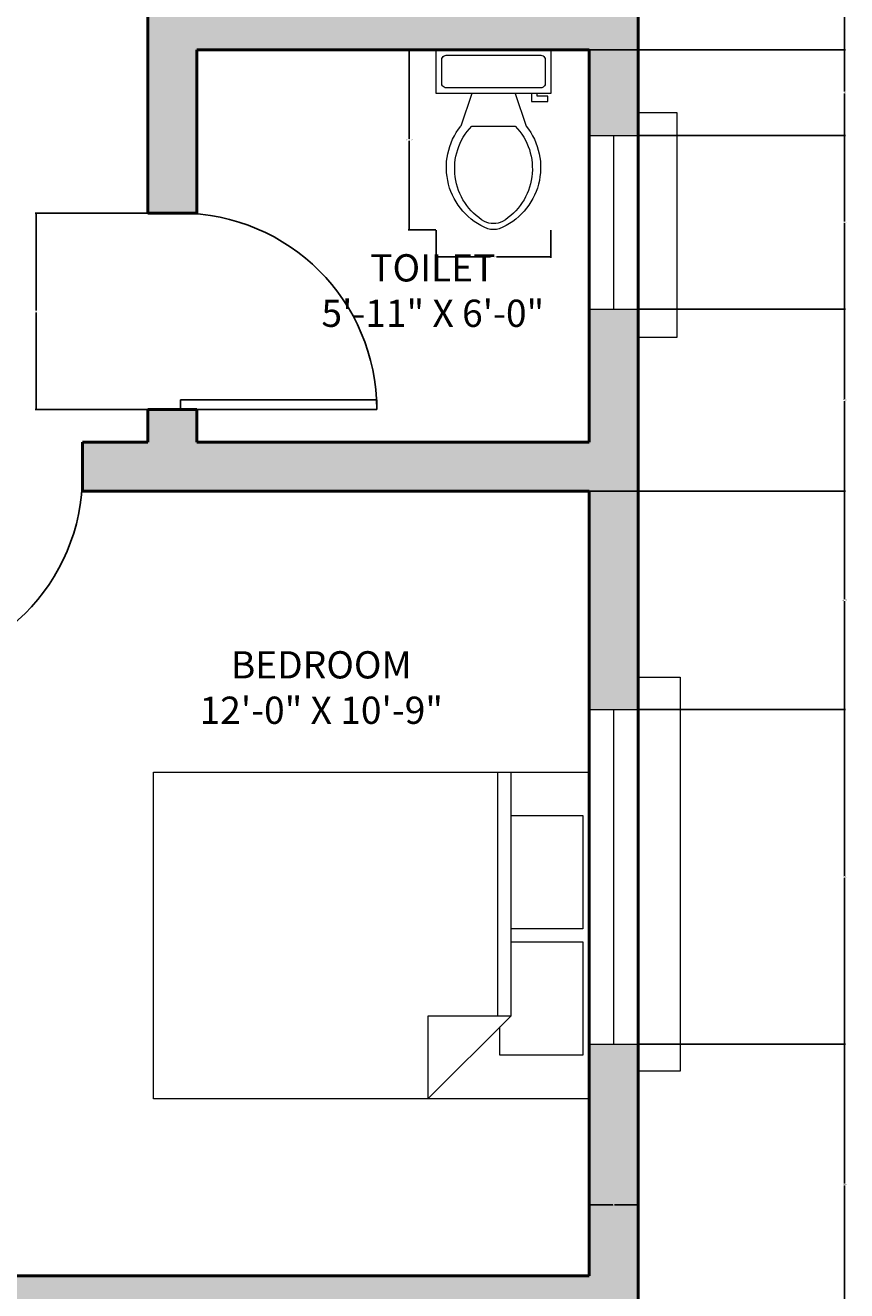
# Model space of a CAD drawing. Units: inches. Extents: x 2710 to 3197, y 524 to 1147.
# Tile 4 of 6: x 3046 to 3197, y 640 to 873. Entities that reach past the tile are written whole.
import ezdxf

# ---------------------------------------------------------------- set-up
doc = ezdxf.new("R2010")
doc.units = ezdxf.units.IN
for name, color, linetype, lineweight in [('A-ANNO-DIMS', 2, 'Continuous', 18), ('A-AREA-IDEN', 7, 'Continuous', 25), ('A-DOOR', 3, 'Continuous', 25), ('A-FLOR-FIXT', 9, 'Continuous', 20), ('A-FURN', 8, 'Continuous', 18), ('A-GLAZ', 4, 'Continuous', 18), ('A-WALL', 7, 'Continuous', 50), ('A-WALL-PATT', 74, 'Continuous', 13)]:
    doc.layers.add(name, color=color, linetype=linetype, lineweight=lineweight)
doc.styles.get("Standard").update_dxf_attribs({"font": 'arial.ttf'})
doc.dimstyles.get("Standard").update_dxf_attribs({"dimtxt": 0.18, "dimasz": 0.18, "dimexe": 0.18, "dimexo": 0.0625, "dimgap": 0.09, "dimtad": 0, "dimtih": 1, "dimtoh": 1, "dimdec": 4, "dimzin": 0, "dimdsep": 46, "dimtxsty": 'Standard', "dimcen": 0.09, "dimadec": 0, "dimazin": 0, "dimtfac": 1, "dimtdec": 4, "dimtofl": 0, "dimtmove": 0, "dimatfit": 3, "dimfxl": 1, "dimtolj": 1, "dimtzin": 0, "dimarcsym": 0})

# ---------------------------------------------------------------- blocks, each defined once
blk = doc.blocks.new('*U8')
for p, q in [((0, 0), (0, 6)), ((36, 0), (36, 6))]:
    blk.add_line(p, q)
blk.add_lwpolyline([(0, 0), (0, -36), (1.75, -36), (1.75, 0)], close=True)
blk.add_arc((0, 0), 36, 270, 0)
blk = doc.blocks.new('*U10')
for p, q in [((0, 0), (0, -6)), ((-36, 0), (-36, -6))]:
    blk.add_line(p, q)
blk.add_lwpolyline([(0, 0), (0, 36), (-1.75, 36), (-1.75, 0)], close=True)
blk.add_arc((0, 0), 36, 90, 180)
blk = doc.blocks.new('Bed - Queen')
for p, q in [((0, -80.00003), (0, 0)), ((0, 0), (59.99999, 0)), ((59.99999, 0), (59.99999, -80.00003)), ((7.99999, -1.2), (28.79998, -1.2)), ((7.99999, -14.4), (7.99999, -1.2)), ((28.79998, -1.2), (28.79998, -14.4)), ((31.19999, -1.2), (51.99999, -1.2)), ((31.19999, -14.4), (31.19999, -1.2)), ((51.99999, -1.2), (51.99999, -16.4)), ((0, -14.4), (44.8, -14.4)), ((59.99999, -29.6), (44.8, -14.4)), ((44.8, -14.4), (44.8, -29.6)), ((44.8, -16.8), (0, -16.8)), ((51.99999, -16.4), (46.79936, -16.4)), ((44.8, -29.6), (59.99999, -29.6)), ((59.99999, -80.00003), (0, -80.00003))]:
    blk.add_line(p, q)
blk = doc.blocks.new('Toilet - top')
for p, q in [((9.5, -6), (9.5, -2)), ((-10, -8.5), (-8, -8.5)), ((-10, -9.5), (-10, -8.5)), ((-8, -8.5), (-8, -8)), ((-7, -8), (-7, -9.5)), ((-4, -8), (-6, -14)), ((4, -8), (6, -14)), ((-7, -9.5), (-10, -9.5)), ((4, -14), (-4, -14))]:
    blk.add_line(p, q)
blk.add_lwpolyline([(10.5, -8), (10.5, 0), (-10.5, 0), (-10.5, -8)], close=True)
for points in [[(-9.5, -2), (-9.5, -6)], [(8.5, -1), (-8.5, -1)], [(-8.5, -7), (8.5, -7)]]:
    blk.add_lwpolyline(points)
for centre, radius, start, end in [((-8.62, -1.88), 0.884, 81.8699, 188.1301), ((8.62, -1.88), 0.884, 351.8699, 98.1301), ((-8.62, -6.12), 0.884, 171.8699, 278.1301), ((8.62, -6.12), 0.884, 261.8699, 8.1301), ((3.52, -21.58), 12.17, 141.4691, 247.9714), ((4.2, -21.82), 11.33, 136.3677, 238.9468), ((-3.52, -21.58), 12.17, 292.0284, 38.5307), ((-4.2, -21.82), 11.33, 301.053, 43.6321), ((0, -27.88), 4, 245.7318, 294.2682), ((0, -29), 4, 254.8605, 285.1395)]:
    blk.add_arc(centre, radius, start, end)
blk = doc.blocks.new('*D24')
at = {"layer": 'A-ANNO-DIMS', "color": 0, "lineweight": -2, "transparency": 16777216}
for p, q in [((3121.22, 868), (3116.14, 868)), ((3116.32, 867.82), (3116.32, 851.66)), ((3116.32, 835.14), (3116.32, 851.3)), ((3121.22, 834.96), (3116.14, 834.96))]:
    blk.add_line(p, q, dxfattribs=at)
at = {"layer": 'A-ANNO-DIMS', "color": 0, "transparency": 16777216}
for points in [[(3116.29, 867.82), (3116.35, 867.82), (3116.32, 868)], [(3116.29, 835.14), (3116.35, 835.14), (3116.32, 834.96)]]:
    blk.add_solid(points, dxfattribs=at)
at = {"layer": 'Defpoints', "color": 0, "transparency": 16777216}
for p in [(3116.32, 868), (3121.28, 868), (3121.28, 834.96)]:
    blk.add_point(p, dxfattribs=at)
at = {"layer": 'A-ANNO-DIMS', "color": 0, "transparency": 16777216, "insert": (3116.32, 851.48), "char_height": 0.18, "attachment_point": 5}
blk.add_mtext('\\A1;WC 33 TYP.', dxfattribs=at)
blk = doc.blocks.new('*D25')
at = {"layer": 'A-ANNO-DIMS', "color": 0, "lineweight": -2, "transparency": 16777216}
for p, q in [((3121.28, 834.89), (3121.28, 829.82)), ((3142.28, 834.89), (3142.28, 829.82)), ((3121.46, 830), (3131.25, 830)), ((3142.1, 830), (3132.31, 830))]:
    blk.add_line(p, q, dxfattribs=at)
at = {"layer": 'A-ANNO-DIMS', "color": 0, "transparency": 16777216}
for points in [[(3121.46, 830.03), (3121.46, 829.97), (3121.28, 830)], [(3142.1, 830.03), (3142.1, 829.97), (3142.28, 830)]]:
    blk.add_solid(points, dxfattribs=at)
at = {"layer": 'Defpoints', "color": 0, "transparency": 16777216}
for p in [(3121.28, 834.96), (3142.28, 834.96), (3121.28, 830)]:
    blk.add_point(p, dxfattribs=at)
at = {"layer": 'A-ANNO-DIMS', "color": 0, "transparency": 16777216, "insert": (3131.78, 830), "char_height": 0.18, "attachment_point": 5}
blk.add_mtext('\\A1;21 TYP.', dxfattribs=at)
blk = doc.blocks.new('*D58')
at = {"layer": 'A-ANNO-DIMS', "color": 0, "lineweight": -2, "transparency": 16777216}
for p, q in [((3158.41, 685.53), (3196.41, 685.53)), ((3196.23, 685.35), (3196.23, 659.95)), ((3196.23, 634.18), (3196.23, 659.59)), ((3149.41, 634), (3196.41, 634))]:
    blk.add_line(p, q, dxfattribs=at)
at = {"layer": 'A-ANNO-DIMS', "color": 0, "transparency": 16777216}
for points in [[(3196.2, 685.35), (3196.26, 685.35), (3196.23, 685.53)], [(3196.2, 634.18), (3196.26, 634.18), (3196.23, 634)]]:
    blk.add_solid(points, dxfattribs=at)
at = {"layer": 'Defpoints', "color": 0, "transparency": 16777216}
for p in [(3158.35, 685.53), (3196.23, 685.53), (3149.35, 634)]:
    blk.add_point(p, dxfattribs=at)
at = {"layer": 'A-ANNO-DIMS', "color": 0, "transparency": 16777216, "insert": (3196.23, 659.77), "char_height": 0.18, "attachment_point": 5}
blk.add_mtext('\\A1;51.53', dxfattribs=at)
blk = doc.blocks.new('*D59')
at = {"layer": 'A-ANNO-DIMS', "color": 0, "lineweight": -2, "transparency": 16777216}
for p, q in [((3158.41, 746.95), (3196.41, 746.95)), ((3196.23, 746.77), (3196.23, 716.42)), ((3196.23, 685.71), (3196.23, 716.06)), ((3158.41, 685.53), (3196.41, 685.53))]:
    blk.add_line(p, q, dxfattribs=at)
at = {"layer": 'A-ANNO-DIMS', "color": 0, "transparency": 16777216}
for points in [[(3196.2, 746.77), (3196.26, 746.77), (3196.23, 746.95)], [(3196.2, 685.71), (3196.26, 685.71), (3196.23, 685.53)]]:
    blk.add_solid(points, dxfattribs=at)
at = {"layer": 'Defpoints', "color": 0, "transparency": 16777216}
for p in [(3158.35, 746.95), (3196.23, 746.95), (3158.35, 685.53)]:
    blk.add_point(p, dxfattribs=at)
at = {"layer": 'A-ANNO-DIMS', "color": 0, "transparency": 16777216, "insert": (3196.23, 716.24), "char_height": 0.18, "attachment_point": 5}
blk.add_mtext('\\A1;61.41', dxfattribs=at)
blk = doc.blocks.new('*D60')
at = {"layer": 'A-ANNO-DIMS', "color": 0, "lineweight": -2, "transparency": 16777216}
for p, q in [((3149.41, 787), (3196.41, 787)), ((3196.23, 786.82), (3196.23, 767.16)), ((3196.23, 747.13), (3196.23, 766.79)), ((3158.41, 746.95), (3196.41, 746.95))]:
    blk.add_line(p, q, dxfattribs=at)
at = {"layer": 'A-ANNO-DIMS', "color": 0, "transparency": 16777216}
for points in [[(3196.2, 786.82), (3196.26, 786.82), (3196.23, 787)], [(3196.2, 747.13), (3196.26, 747.13), (3196.23, 746.95)]]:
    blk.add_solid(points, dxfattribs=at)
at = {"layer": 'Defpoints', "color": 0, "transparency": 16777216}
for p in [(3149.35, 787), (3196.23, 787), (3158.35, 746.95)]:
    blk.add_point(p, dxfattribs=at)
at = {"layer": 'A-ANNO-DIMS', "color": 0, "transparency": 16777216, "insert": (3196.23, 766.97), "char_height": 0.18, "attachment_point": 5}
blk.add_mtext('\\A1;40.055', dxfattribs=at)
blk = doc.blocks.new('*D61')
at = {"layer": 'A-ANNO-DIMS', "color": 0, "lineweight": -2, "transparency": 16777216}
for p, q in [((3158.41, 820.38), (3196.41, 820.38)), ((3196.23, 820.2), (3196.23, 803.87)), ((3196.23, 787.18), (3196.23, 803.51)), ((3149.41, 787), (3196.41, 787))]:
    blk.add_line(p, q, dxfattribs=at)
at = {"layer": 'A-ANNO-DIMS', "color": 0, "transparency": 16777216}
for points in [[(3196.2, 820.2), (3196.26, 820.2), (3196.23, 820.38)], [(3196.2, 787.18), (3196.26, 787.18), (3196.23, 787)]]:
    blk.add_solid(points, dxfattribs=at)
at = {"layer": 'Defpoints', "color": 0, "transparency": 16777216}
for p in [(3158.35, 820.38), (3196.23, 820.38), (3149.35, 787)]:
    blk.add_point(p, dxfattribs=at)
at = {"layer": 'A-ANNO-DIMS', "color": 0, "transparency": 16777216, "insert": (3196.23, 803.69), "char_height": 0.18, "attachment_point": 5}
blk.add_mtext('\\A1;33.38', dxfattribs=at)
blk = doc.blocks.new('*D62')
at = {"layer": 'A-ANNO-DIMS', "color": 0, "lineweight": -2, "transparency": 16777216}
for p, q in [((3158.41, 852.3), (3196.41, 852.3)), ((3196.23, 852.12), (3196.23, 836.52)), ((3196.23, 820.56), (3196.23, 836.16)), ((3158.41, 820.38), (3196.41, 820.38))]:
    blk.add_line(p, q, dxfattribs=at)
at = {"layer": 'A-ANNO-DIMS', "color": 0, "transparency": 16777216}
for points in [[(3196.2, 852.12), (3196.26, 852.12), (3196.23, 852.3)], [(3196.2, 820.56), (3196.26, 820.56), (3196.23, 820.38)]]:
    blk.add_solid(points, dxfattribs=at)
at = {"layer": 'Defpoints', "color": 0, "transparency": 16777216}
for p in [(3158.35, 852.3), (3196.23, 852.3), (3158.35, 820.38)]:
    blk.add_point(p, dxfattribs=at)
at = {"layer": 'A-ANNO-DIMS', "color": 0, "transparency": 16777216, "insert": (3196.23, 836.34), "char_height": 0.18, "attachment_point": 5}
blk.add_mtext('\\A1;31.92', dxfattribs=at)
blk = doc.blocks.new('*D63')
at = {"layer": 'A-ANNO-DIMS', "color": 0, "lineweight": -2, "transparency": 16777216}
for p, q in [((3149.41, 868), (3196.41, 868)), ((3196.23, 867.82), (3196.23, 860.33)), ((3196.23, 852.48), (3196.23, 859.97)), ((3158.41, 852.3), (3196.41, 852.3))]:
    blk.add_line(p, q, dxfattribs=at)
at = {"layer": 'A-ANNO-DIMS', "color": 0, "transparency": 16777216}
for points in [[(3196.2, 867.82), (3196.26, 867.82), (3196.23, 868)], [(3196.2, 852.48), (3196.26, 852.48), (3196.23, 852.3)]]:
    blk.add_solid(points, dxfattribs=at)
at = {"layer": 'Defpoints', "color": 0, "transparency": 16777216}
for p in [(3149.35, 868), (3196.23, 868), (3158.35, 852.3)]:
    blk.add_point(p, dxfattribs=at)
at = {"layer": 'A-ANNO-DIMS', "color": 0, "transparency": 16777216, "insert": (3196.23, 860.15), "char_height": 0.18, "attachment_point": 5}
blk.add_mtext('\\A1;15.7', dxfattribs=at)
blk = doc.blocks.new('*D64')
at = {"layer": 'A-ANNO-DIMS', "color": 0, "lineweight": -2, "transparency": 16777216}
for p, q in [((3158.41, 905.22), (3196.41, 905.22)), ((3196.23, 905.04), (3196.23, 886.79)), ((3196.23, 868.18), (3196.23, 886.43)), ((3149.41, 868), (3196.41, 868))]:
    blk.add_line(p, q, dxfattribs=at)
at = {"layer": 'A-ANNO-DIMS', "color": 0, "transparency": 16777216}
for points in [[(3196.2, 905.04), (3196.26, 905.04), (3196.23, 905.22)], [(3196.2, 868.18), (3196.26, 868.18), (3196.23, 868)]]:
    blk.add_solid(points, dxfattribs=at)
at = {"layer": 'Defpoints', "color": 0, "transparency": 16777216}
for p in [(3158.35, 905.22), (3196.23, 905.22), (3149.35, 868)]:
    blk.add_point(p, dxfattribs=at)
at = {"layer": 'A-ANNO-DIMS', "color": 0, "transparency": 16777216, "insert": (3196.23, 886.61), "char_height": 0.18, "attachment_point": 5}
blk.add_mtext('\\A1;37.22', dxfattribs=at)
blk = doc.blocks.new('*D76')
at = {"layer": 'A-ANNO-DIMS', "color": 0, "lineweight": -2, "transparency": 16777216}
for p, q in [((3077.29, 838), (3047.67, 838)), ((3047.85, 837.82), (3047.85, 820.18)), ((3047.85, 802.18), (3047.85, 819.82)), ((3077.29, 802), (3047.67, 802))]:
    blk.add_line(p, q, dxfattribs=at)
at = {"layer": 'A-ANNO-DIMS', "color": 0, "transparency": 16777216}
for points in [[(3047.82, 837.82), (3047.88, 837.82), (3047.85, 838)], [(3047.82, 802.18), (3047.88, 802.18), (3047.85, 802)]]:
    blk.add_solid(points, dxfattribs=at)
at = {"layer": 'Defpoints', "color": 0, "transparency": 16777216}
for p in [(3047.85, 838), (3077.35, 838), (3077.35, 802)]:
    blk.add_point(p, dxfattribs=at)
at = {"layer": 'A-ANNO-DIMS', "color": 0, "transparency": 16777216, "insert": (3047.85, 820), "char_height": 0.18, "attachment_point": 5}
blk.add_mtext('\\A1;36', dxfattribs=at)
blk = doc.blocks.new('*D78')
at = {"layer": 'A-ANNO-DIMS', "color": 0, "lineweight": -2, "transparency": 16777216}
for p, q in [((3149.35, 685.47), (3149.35, 655.85)), ((3158.35, 685.47), (3158.35, 655.85)), ((3149.53, 656.03), (3153.7, 656.03)), ((3158.17, 656.03), (3154, 656.03))]:
    blk.add_line(p, q, dxfattribs=at)
at = {"layer": 'A-ANNO-DIMS', "color": 0, "transparency": 16777216}
for points in [[(3149.53, 656.06), (3149.53, 656), (3149.35, 656.03)], [(3158.17, 656.06), (3158.17, 656), (3158.35, 656.03)]]:
    blk.add_solid(points, dxfattribs=at)
at = {"layer": 'Defpoints', "color": 0, "transparency": 16777216}
for p in [(3149.35, 685.53), (3158.35, 685.53), (3149.35, 656.03)]:
    blk.add_point(p, dxfattribs=at)
at = {"layer": 'A-ANNO-DIMS', "color": 0, "transparency": 16777216, "insert": (3153.85, 656.03), "char_height": 0.18, "attachment_point": 5}
blk.add_mtext('\\A1;9', dxfattribs=at)

msp = doc.modelspace()

# ---------------------------------------------------------------- hatches: boundary and pattern name
at = {"layer": 'A-WALL-PATT'}
h = msp.add_hatch(color=256, dxfattribs=at)
h.dxf.hatch_style = 1
h.paths.add_polyline_path([(2898.3484, 1096.0017), (2898.3484, 967.0017), (2948.3484, 967.0017), (2948.3484, 787.0017), (2957.3484, 787.0017), (2957.3484, 793.0017), (2957.3484, 833.0017), (2957.3484, 967.0017), (3007.3484, 967.0017), (3007.3484, 973.0017), (3007.3484, 1009.0017), (3007.3484, 1096.0017), (3149.3484, 1096.0017), (3149.3484, 1084.4601), (3158.3484, 1084.4601), (3158.3484, 1105.0017), (2991.781, 1105.0017), (2991.781, 1096.0017), (2998.3484, 1096.0017), (2998.3484, 976.0017), (2957.3484, 976.0017), (2957.3484, 1003.0017), (2966.3484, 1003.0017), (2966.3484, 1012.0017), (2957.3484, 1012.0017), (2957.3484, 1096.0017), (2963.4487, 1096.0017), (2963.4487, 1105.0017), (2940.703, 1105.0017), (2940.703, 1096.0017), (2948.3484, 1096.0017), (2948.3484, 1012.0017), (2939.3484, 1012.0017), (2939.3484, 1003.0017), (2948.3484, 1003.0017), (2948.3484, 976.0017), (2907.3484, 976.0017), (2907.3484, 1096.0017), (2916.9598, 1096.0017), (2916.9598, 1105.0017), (2857.03, 1105.0017), (2857.03, 1096.0017)])
h.paths.add_polyline_path([(2789.8274, 1096.0017), (2789.8274, 1105.0017), (2747.3484, 1105.0017), (2747.3484, 943.327), (2756.3484, 943.327), (2756.3484, 967.0017), (2828.3484, 967.0017), (2828.3484, 909.0017), (2837.3484, 909.0017), (2837.3484, 967.0017), (2862.3484, 967.0017), (2862.3484, 973.0017), (2862.3484, 976.0017), (2756.3484, 976.0017), (2756.3484, 1096.0017)])
h.paths.add_polyline_path([(2828.3484, 868.0017), (2828.3484, 830.0017), (2837.3484, 830.0017), (2837.3484, 877.0017), (2756.3484, 877.0017), (2756.3484, 904.8338), (2747.3484, 904.8338), (2747.3484, 858.8554), (2756.3484, 858.8554), (2756.3484, 868.0017)])
h.paths.add_polyline_path([(2747.3484, 742.5572), (2756.3484, 742.5572), (2756.3484, 787.0017), (2849.3484, 787.0017), (2849.3484, 796.0017), (2837.3484, 796.0017), (2837.3484, 802.0017), (2831.3484, 802.0017), (2828.3484, 802.0017), (2828.3484, 796.0017), (2756.3484, 796.0017), (2756.3484, 819.3052), (2747.3484, 819.3052)])
h.paths.add_polyline_path([(2756.3484, 643.0017), (2756.3484, 672.4477), (2747.3484, 672.4477), (2747.3484, 565.0017), (2825.5051, 565.0017), (2825.5051, 574.0017), (2756.3484, 574.0017), (2756.3484, 634.0017), (2891.3484, 634.0017), (2891.3484, 787.0017), (2908.3484, 787.0017), (2908.3484, 793.0017), (2908.3484, 796.0017), (2891.3484, 796.0017), (2885.3484, 796.0017), (2885.3484, 790.0017), (2885.3484, 754.0017), (2885.3484, 643.0017)])
h.paths.add_polyline_path([(2924.8484, 565.0017), (2924.8484, 571.0017), (2924.8484, 574.0017), (2872.3715, 574.0017), (2872.3715, 565.0017)])
h.paths.add_polyline_path([(2984.8484, 574.0017), (2984.8484, 571.0017), (2984.8484, 565.0017), (3050.793, 565.0017), (3050.793, 574.0017)])
h.paths.add_polyline_path([(3158.3484, 565.0017), (3158.3484, 685.5326), (3149.3484, 685.5326), (3149.3484, 675.4542), (3149.3484, 643.0017), (3020.3484, 643.0017), (3020.3484, 796.0017), (3014.3484, 796.0017), (2997.3484, 796.0017), (2997.3484, 787.0017), (3014.3484, 787.0017), (3014.3484, 634.0017), (3149.3484, 634.0017), (3149.3484, 574.0017), (3104.3903, 574.0017), (3104.3903, 565.0017)])
h.paths.add_polyline_path([(3149.3484, 787.0017), (3149.3484, 746.9465), (3158.3484, 746.9465), (3158.3484, 820.3805), (3149.3484, 820.3805), (3149.3484, 796.0017), (3077.3484, 796.0017), (3077.3484, 802.0017), (3074.3484, 802.0017), (3068.3484, 802.0017), (3068.3484, 796.0017), (3056.3484, 796.0017), (3056.3484, 790.0017), (3056.3484, 787.0017)])
h.paths.add_polyline_path([(3158.3484, 905.224), (3149.3484, 905.224), (3149.3484, 877.0017), (3068.3484, 877.0017), (3068.3484, 838.0017), (3074.3484, 838.0017), (3077.3484, 838.0017), (3077.3484, 868.0017), (3149.3484, 868.0017), (3149.3484, 852.3022), (3158.3484, 852.3022)], flags=17)
h.paths.add_polyline_path([(3099.2867, 814.3126), (3142.0289, 814.3126), (3142.0289, 832.97), (3099.2867, 832.97)], flags=25)
h.paths.add_polyline_path([(2981.8144, 832.8032), (3033.605, 832.8032), (3033.605, 851.4605), (2981.8144, 851.4605)], flags=25)

# ---------------------------------------------------------------- linework, layer by layer
at = {"layer": 'A-GLAZ'}
for p, q in [((3158.3484, 856.5165), (3165.411, 856.5165)), ((3165.411, 856.5165), (3165.411, 815.192)), ((3149.3484, 852.3022), (3158.3484, 852.3022)), ((3153.8484, 820.3805), (3153.8484, 852.3022)), ((3149.3484, 820.3805), (3158.3484, 820.3805)), ((3165.411, 815.192), (3158.3484, 815.192)), ((3158.3484, 752.8808), (3166.0509, 752.8808)), ((3166.0509, 752.8808), (3166.0509, 680.5575)), ((3149.3484, 746.9465), (3158.3484, 746.9465)), ((3153.8484, 685.5326), (3153.8484, 746.9465)), ((3149.3484, 685.5326), (3158.3484, 685.5326)), ((3166.0509, 680.5575), (3158.3484, 680.5575))]:
    msp.add_line(p, q, dxfattribs=at)
at = {"layer": 'A-WALL'}
for p, q in [((3158.3484, 565.0017), (3158.3484, 1105.0017)), ((3068.3484, 838.0017), (3068.3484, 877.0017)), ((3149.3484, 868.0017), (3077.3484, 868.0017)), ((3077.3484, 838.0017), (3077.3484, 868.0017)), ((3149.3484, 796.0017), (3149.3484, 868.0017)), ((3068.3484, 838.0017), (3077.3484, 838.0017)), ((3068.3484, 796.0017), (3068.3484, 802.0017)), ((3068.3484, 802.0017), (3077.3484, 802.0017)), ((3077.3484, 796.0017), (3077.3484, 802.0017)), ((3056.3484, 796.0017), (3056.3484, 787.0017)), ((3068.3484, 796.0017), (3056.3484, 796.0017)), ((3149.3484, 796.0017), (3077.3484, 796.0017)), ((3149.3484, 787.0017), (3056.3484, 787.0017)), ((3149.3484, 643.0017), (3149.3484, 787.0017)), ((3149.3484, 643.0017), (3020.3484, 643.0017))]:
    msp.add_line(p, q, dxfattribs=at)

# ---------------------------------------------------------------- block references
at = {"layer": 'A-DOOR', "rotation": 270}
msp.add_blockref('*U10', (3074.3484, 802.0017), dxfattribs=at)
at = {"layer": 'A-DOOR'}
msp.add_blockref('*U8', (3020.3484, 790.0017), dxfattribs=at)
at = {"layer": 'A-FLOR-FIXT', "xscale": -1}
msp.add_blockref('Toilet - top', (3131.7806, 868.0017), dxfattribs=at)
at = {"layer": 'A-FURN', "rotation": 270}
msp.add_blockref('Bed - Queen', (3149.3484, 735.4541), dxfattribs=at)

# ---------------------------------------------------------------- texts
at = {"layer": 'A-AREA-IDEN', "char_height": 5, "attachment_point": 1}
for s, insert in [('\\pxqc;TOILET\\P5\'-11" X 6\'-0"', (3091.8111, 830.4853)), ('\\pxqc;BEDROOM\\P12\'-0" X 10\'-9"', (3071.3399, 757.6252))]:
    msp.add_mtext_dynamic_manual_height_columns(s, width=57.655828, gutter_width=12.5, heights=[0], dxfattribs=dict(at, insert=insert))

# ---------------------------------------------------------------- dimensions: what is measured, and where the dimension line sits
at = {"layer": 'A-ANNO-DIMS'}
for base, p1, p2, angle, override, picture, middle in [((3196.2275, 905.224), (3149.3484, 868.0017), (3158.3484, 905.224), 90, {"dimdec": 2, "dimlfac": 1, "dimrnd": 0, "dimzin": 0, "dimdsep": 46, "dimlunit": 2}, '*D64', (3196.2275, 886.6129)), ((3196.2275, 868.0017), (3158.3484, 852.3022), (3149.3484, 868.0017), 90, {"dimdec": 1, "dimlfac": 1, "dimrnd": 0, "dimzin": 0, "dimdsep": 46, "dimlunit": 2}, '*D63', (3196.2275, 860.1519)), ((3196.2275, 852.3022), (3158.3484, 820.3805), (3158.3484, 852.3022), 90, {"dimdec": 2, "dimlfac": 1, "dimrnd": 0, "dimzin": 0, "dimdsep": 46, "dimlunit": 2}, '*D62', (3196.2275, 836.3414)), ((3047.8484, 838.0017), (3077.3484, 802.0017), (3077.3484, 838.0017), 90, {"dimdec": 0, "dimlfac": 1, "dimrnd": 0, "dimzin": 0, "dimdsep": 46, "dimlunit": 2}, '*D76', (3047.8484, 820.0017)), ((3196.2275, 820.3805), (3149.3484, 787.0017), (3158.3484, 820.3805), 90, {"dimdec": 2, "dimlfac": 1, "dimrnd": 0, "dimzin": 0, "dimdsep": 46, "dimlunit": 2}, '*D61', (3196.2275, 803.6911)), ((3196.2275, 787.0017), (3158.3484, 746.9465), (3149.3484, 787.0017), 90, {"dimdec": 3, "dimlfac": 1, "dimrnd": 0, "dimzin": 0, "dimdsep": 46, "dimlunit": 2}, '*D60', (3196.2275, 766.9741)), ((3196.2275, 746.9465), (3158.3484, 685.5326), (3158.3484, 746.9465), 90, {"dimdec": 2, "dimlfac": 1, "dimrnd": 0, "dimzin": 0, "dimdsep": 46, "dimlunit": 2}, '*D59', (3196.2275, 716.2395)), ((3196.2275, 685.5326), (3149.3484, 634.0017), (3158.3484, 685.5326), 90, {"dimdec": 2, "dimlfac": 1, "dimrnd": 0, "dimzin": 0, "dimdsep": 46, "dimlunit": 2}, '*D58', (3196.2275, 659.7671)), ((3149.3484, 656.0326), (3158.3484, 685.5326), (3149.3484, 685.5326), 180, {"dimdec": 0, "dimlfac": 1, "dimrnd": 0, "dimzin": 0, "dimdsep": 46, "dimlunit": 2}, '*D78', (3153.8484, 656.0326))]:
    dim = msp.add_linear_dim(base=base, p1=p1, p2=p2, angle=angle, dimstyle='Standard', override=override, dxfattribs=at)
    dim.commit()
    dim.dimension.update_dxf_attribs({"geometry": picture, "text_midpoint": middle})
for base, p1, p2, angle, text, picture, middle in [((3116.3236, 868.0017), (3121.2806, 834.9554), (3121.2806, 868.0017), 90, 'WC <> TYP.', '*D24', (3116.3236, 851.4785)), ((3121.2806, 829.9985), (3142.2806, 834.9554), (3121.2806, 834.9554), 180, '<> TYP.', '*D25', (3131.7806, 829.9985))]:
    dim = msp.add_linear_dim(base=base, p1=p1, p2=p2, angle=angle, text=text, dimstyle='Standard', override={"dimdec": 0, "dimlfac": 1, "dimrnd": 0, "dimzin": 0, "dimdsep": 46, "dimlunit": 2}, dxfattribs=at)
    dim.commit()
    dim.dimension.update_dxf_attribs({"geometry": picture, "text_midpoint": middle})

doc.saveas('drawing.dxf')
